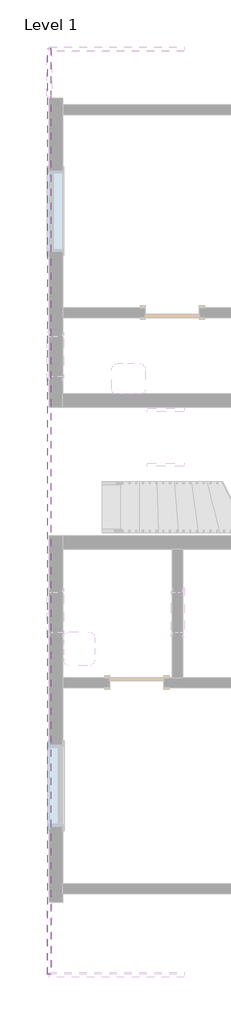
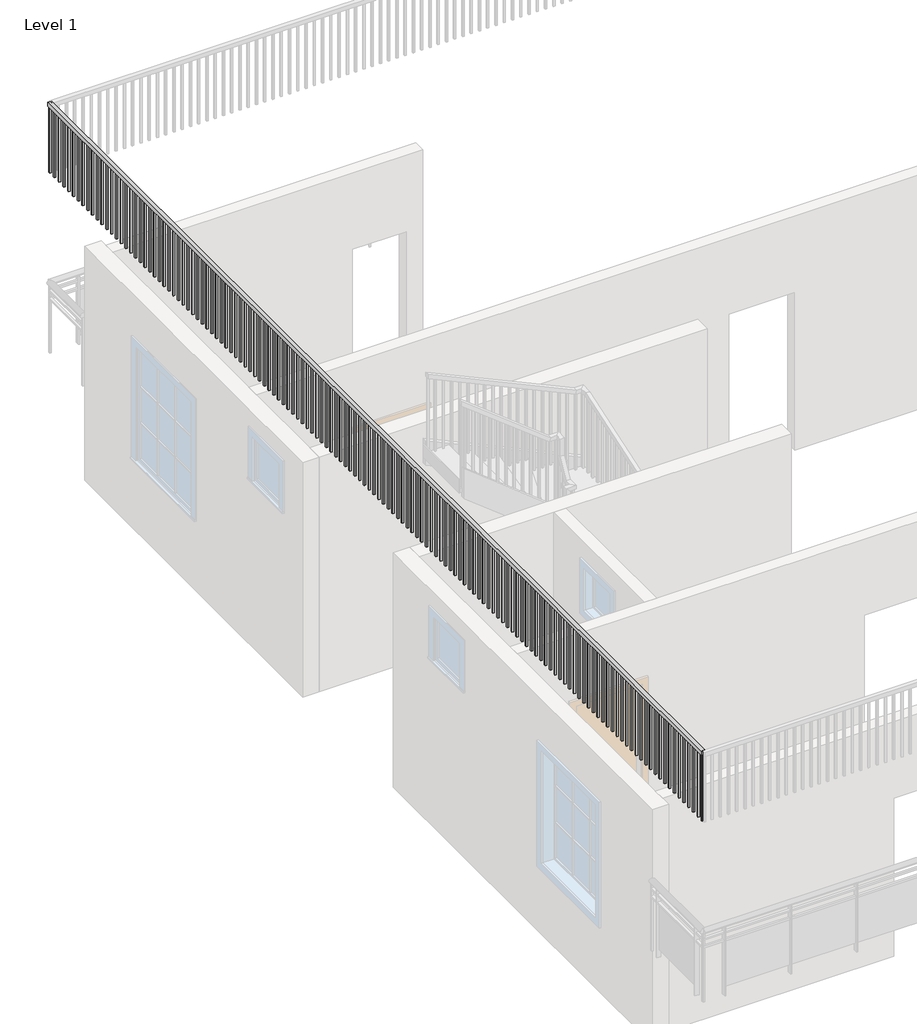
# One storey, part 3 of 7: 1 railing.
"""IFC4 building model written with IfcOpenShell, lengths in millimetres."""

from ifc_helpers import new_model, si_unit, frame, origin, place, context, project, spatial, polyline, outline, extrude, element, save

model = new_model("IFC4")

# Units and contexts
model_context = context("Model", 3, world=origin())
ifc_project = project(units=[si_unit("LENGTHUNIT", "METRE", prefix="MILLI")], contexts=[model_context])

# Site, building, storey
site = spatial("IfcSite", under=ifc_project)
building = spatial("IfcBuilding", under=site)
storey = spatial("IfcBuildingStorey", under=building, Name="Level 1", Elevation=0.0)

# Railing
placement = place(None, origin())
element("IfcRailing", 1, ObjectType="Handrail - Rectangular", at=placement, inside=storey, context=model_context, shape_type="SweptSolid", body=[
    extrude(outline(polyline([(-8502.50975, 12460.2089473), (-8451.70975, 12460.2089473), (-8451.70975, -1458.9910527), (-8502.50975, -1458.9910527), (-8502.50975, 12460.2089473)])), frame((0.0, 0.0, 4419.6), z_axis=(0.0, 0.0, 1.0), x_axis=(1.0, 0.0, 0.0)), (0.0, 0.0, 1.0), 50.8),
    extrude(outline(polyline([(-8486.63475, -1347.8660527), (-8467.58475, -1347.8660527), (-8467.58475, -1366.9160527), (-8486.63475, -1366.9160527), (-8486.63475, -1347.8660527)])), frame((0.0, 0.0, 3556.0), z_axis=(0.0, 0.0, 1.0), x_axis=(1.0, 0.0, 0.0)), (0.0, 0.0, 1.0), 863.6),
    extrude(outline(polyline([(-8486.63475, -1246.2660527), (-8467.58475, -1246.2660527), (-8467.58475, -1265.3160527), (-8486.63475, -1265.3160527), (-8486.63475, -1246.2660527)])), frame((0.0, 0.0, 3556.0), z_axis=(0.0, 0.0, 1.0), x_axis=(1.0, 0.0, 0.0)), (0.0, 0.0, 1.0), 863.6),
    extrude(outline(polyline([(-8486.63475, -1144.6660527), (-8467.58475, -1144.6660527), (-8467.58475, -1163.7160527), (-8486.63475, -1163.7160527), (-8486.63475, -1144.6660527)])), frame((0.0, 0.0, 3556.0), z_axis=(0.0, 0.0, 1.0), x_axis=(1.0, 0.0, 0.0)), (0.0, 0.0, 1.0), 863.6),
    extrude(outline(polyline([(-8486.63475, -1043.0660527), (-8467.58475, -1043.0660527), (-8467.58475, -1062.1160527), (-8486.63475, -1062.1160527), (-8486.63475, -1043.0660527)])), frame((0.0, 0.0, 3556.0), z_axis=(0.0, 0.0, 1.0), x_axis=(1.0, 0.0, 0.0)), (0.0, 0.0, 1.0), 863.6),
    extrude(outline(polyline([(-8486.63475, -941.4660527), (-8467.58475, -941.4660527), (-8467.58475, -960.5160527), (-8486.63475, -960.5160527), (-8486.63475, -941.4660527)])), frame((0.0, 0.0, 3556.0), z_axis=(0.0, 0.0, 1.0), x_axis=(1.0, 0.0, 0.0)), (0.0, 0.0, 1.0), 863.6),
    extrude(outline(polyline([(-8486.63475, -839.8660527), (-8467.58475, -839.8660527), (-8467.58475, -858.9160527), (-8486.63475, -858.9160527), (-8486.63475, -839.8660527)])), frame((0.0, 0.0, 3556.0), z_axis=(0.0, 0.0, 1.0), x_axis=(1.0, 0.0, 0.0)), (0.0, 0.0, 1.0), 863.6),
    extrude(outline(polyline([(-8486.63475, -738.2660527), (-8467.58475, -738.2660527), (-8467.58475, -757.3160527), (-8486.63475, -757.3160527), (-8486.63475, -738.2660527)])), frame((0.0, 0.0, 3556.0), z_axis=(0.0, 0.0, 1.0), x_axis=(1.0, 0.0, 0.0)), (0.0, 0.0, 1.0), 863.6),
    extrude(outline(polyline([(-8486.63475, -636.6660527), (-8467.58475, -636.6660527), (-8467.58475, -655.7160527), (-8486.63475, -655.7160527), (-8486.63475, -636.6660527)])), frame((0.0, 0.0, 3556.0), z_axis=(0.0, 0.0, 1.0), x_axis=(1.0, 0.0, 0.0)), (0.0, 0.0, 1.0), 863.6),
    extrude(outline(polyline([(-8486.63475, -535.0660527), (-8467.58475, -535.0660527), (-8467.58475, -554.1160527), (-8486.63475, -554.1160527), (-8486.63475, -535.0660527)])), frame((0.0, 0.0, 3556.0), z_axis=(0.0, 0.0, 1.0), x_axis=(1.0, 0.0, 0.0)), (0.0, 0.0, 1.0), 863.6),
    extrude(outline(polyline([(-8486.63475, -433.4660527), (-8467.58475, -433.4660527), (-8467.58475, -452.5160527), (-8486.63475, -452.5160527), (-8486.63475, -433.4660527)])), frame((0.0, 0.0, 3556.0), z_axis=(0.0, 0.0, 1.0), x_axis=(1.0, 0.0, 0.0)), (0.0, 0.0, 1.0), 863.6),
    extrude(outline(polyline([(-8486.63475, -331.8660527), (-8467.58475, -331.8660527), (-8467.58475, -350.9160527), (-8486.63475, -350.9160527), (-8486.63475, -331.8660527)])), frame((0.0, 0.0, 3556.0), z_axis=(0.0, 0.0, 1.0), x_axis=(1.0, 0.0, 0.0)), (0.0, 0.0, 1.0), 863.6),
    extrude(outline(polyline([(-8486.63475, -230.2660527), (-8467.58475, -230.2660527), (-8467.58475, -249.3160527), (-8486.63475, -249.3160527), (-8486.63475, -230.2660527)])), frame((0.0, 0.0, 3556.0), z_axis=(0.0, 0.0, 1.0), x_axis=(1.0, 0.0, 0.0)), (0.0, 0.0, 1.0), 863.6),
    extrude(outline(polyline([(-8486.63475, -128.6660527), (-8467.58475, -128.6660527), (-8467.58475, -147.7160527), (-8486.63475, -147.7160527), (-8486.63475, -128.6660527)])), frame((0.0, 0.0, 3556.0), z_axis=(0.0, 0.0, 1.0), x_axis=(1.0, 0.0, 0.0)), (0.0, 0.0, 1.0), 863.6),
    extrude(outline(polyline([(-8486.63475, -27.0660527), (-8467.58475, -27.0660527), (-8467.58475, -46.1160527), (-8486.63475, -46.1160527), (-8486.63475, -27.0660527)])), frame((0.0, 0.0, 3556.0), z_axis=(0.0, 0.0, 1.0), x_axis=(1.0, 0.0, 0.0)), (0.0, 0.0, 1.0), 863.6),
    extrude(outline(polyline([(-8486.63475, 74.5339473), (-8467.58475, 74.5339473), (-8467.58475, 55.4839473), (-8486.63475, 55.4839473), (-8486.63475, 74.5339473)])), frame((0.0, 0.0, 3556.0), z_axis=(0.0, 0.0, 1.0), x_axis=(1.0, 0.0, 0.0)), (0.0, 0.0, 1.0), 863.6),
    extrude(outline(polyline([(-8486.63475, 176.1339473), (-8467.58475, 176.1339473), (-8467.58475, 157.0839473), (-8486.63475, 157.0839473), (-8486.63475, 176.1339473)])), frame((0.0, 0.0, 3556.0), z_axis=(0.0, 0.0, 1.0), x_axis=(1.0, 0.0, 0.0)), (0.0, 0.0, 1.0), 863.6),
    extrude(outline(polyline([(-8486.63475, 277.7339473), (-8467.58475, 277.7339473), (-8467.58475, 258.6839473), (-8486.63475, 258.6839473), (-8486.63475, 277.7339473)])), frame((0.0, 0.0, 3556.0), z_axis=(0.0, 0.0, 1.0), x_axis=(1.0, 0.0, 0.0)), (0.0, 0.0, 1.0), 863.6),
    extrude(outline(polyline([(-8486.63475, 379.3339473), (-8467.58475, 379.3339473), (-8467.58475, 360.2839473), (-8486.63475, 360.2839473), (-8486.63475, 379.3339473)])), frame((0.0, 0.0, 3556.0), z_axis=(0.0, 0.0, 1.0), x_axis=(1.0, 0.0, 0.0)), (0.0, 0.0, 1.0), 863.6),
    extrude(outline(polyline([(-8486.63475, 480.9339473), (-8467.58475, 480.9339473), (-8467.58475, 461.8839473), (-8486.63475, 461.8839473), (-8486.63475, 480.9339473)])), frame((0.0, 0.0, 3556.0), z_axis=(0.0, 0.0, 1.0), x_axis=(1.0, 0.0, 0.0)), (0.0, 0.0, 1.0), 863.6),
    extrude(outline(polyline([(-8486.63475, 582.5339473), (-8467.58475, 582.5339473), (-8467.58475, 563.4839473), (-8486.63475, 563.4839473), (-8486.63475, 582.5339473)])), frame((0.0, 0.0, 3556.0), z_axis=(0.0, 0.0, 1.0), x_axis=(1.0, 0.0, 0.0)), (0.0, 0.0, 1.0), 863.6),
    extrude(outline(polyline([(-8486.63475, 684.1339473), (-8467.58475, 684.1339473), (-8467.58475, 665.0839473), (-8486.63475, 665.0839473), (-8486.63475, 684.1339473)])), frame((0.0, 0.0, 3556.0), z_axis=(0.0, 0.0, 1.0), x_axis=(1.0, 0.0, 0.0)), (0.0, 0.0, 1.0), 863.6),
    extrude(outline(polyline([(-8486.63475, 785.7339473), (-8467.58475, 785.7339473), (-8467.58475, 766.6839473), (-8486.63475, 766.6839473), (-8486.63475, 785.7339473)])), frame((0.0, 0.0, 3556.0), z_axis=(0.0, 0.0, 1.0), x_axis=(1.0, 0.0, 0.0)), (0.0, 0.0, 1.0), 863.6),
    extrude(outline(polyline([(-8486.63475, 887.3339473), (-8467.58475, 887.3339473), (-8467.58475, 868.2839473), (-8486.63475, 868.2839473), (-8486.63475, 887.3339473)])), frame((0.0, 0.0, 3556.0), z_axis=(0.0, 0.0, 1.0), x_axis=(1.0, 0.0, 0.0)), (0.0, 0.0, 1.0), 863.6),
    extrude(outline(polyline([(-8486.63475, 988.9339473), (-8467.58475, 988.9339473), (-8467.58475, 969.8839473), (-8486.63475, 969.8839473), (-8486.63475, 988.9339473)])), frame((0.0, 0.0, 3556.0), z_axis=(0.0, 0.0, 1.0), x_axis=(1.0, 0.0, 0.0)), (0.0, 0.0, 1.0), 863.6),
    extrude(outline(polyline([(-8486.63475, 1090.5339473), (-8467.58475, 1090.5339473), (-8467.58475, 1071.4839473), (-8486.63475, 1071.4839473), (-8486.63475, 1090.5339473)])), frame((0.0, 0.0, 3556.0), z_axis=(0.0, 0.0, 1.0), x_axis=(1.0, 0.0, 0.0)), (0.0, 0.0, 1.0), 863.6),
    extrude(outline(polyline([(-8486.63475, 1192.1339473), (-8467.58475, 1192.1339473), (-8467.58475, 1173.0839473), (-8486.63475, 1173.0839473), (-8486.63475, 1192.1339473)])), frame((0.0, 0.0, 3556.0), z_axis=(0.0, 0.0, 1.0), x_axis=(1.0, 0.0, 0.0)), (0.0, 0.0, 1.0), 863.6),
    extrude(outline(polyline([(-8486.63475, 1293.7339473), (-8467.58475, 1293.7339473), (-8467.58475, 1274.6839473), (-8486.63475, 1274.6839473), (-8486.63475, 1293.7339473)])), frame((0.0, 0.0, 3556.0), z_axis=(0.0, 0.0, 1.0), x_axis=(1.0, 0.0, 0.0)), (0.0, 0.0, 1.0), 863.6),
    extrude(outline(polyline([(-8486.63475, 1395.3339473), (-8467.58475, 1395.3339473), (-8467.58475, 1376.2839473), (-8486.63475, 1376.2839473), (-8486.63475, 1395.3339473)])), frame((0.0, 0.0, 3556.0), z_axis=(0.0, 0.0, 1.0), x_axis=(1.0, 0.0, 0.0)), (0.0, 0.0, 1.0), 863.6),
    extrude(outline(polyline([(-8486.63475, 1496.9339473), (-8467.58475, 1496.9339473), (-8467.58475, 1477.8839473), (-8486.63475, 1477.8839473), (-8486.63475, 1496.9339473)])), frame((0.0, 0.0, 3556.0), z_axis=(0.0, 0.0, 1.0), x_axis=(1.0, 0.0, 0.0)), (0.0, 0.0, 1.0), 863.6),
    extrude(outline(polyline([(-8486.63475, 1598.5339473), (-8467.58475, 1598.5339473), (-8467.58475, 1579.4839473), (-8486.63475, 1579.4839473), (-8486.63475, 1598.5339473)])), frame((0.0, 0.0, 3556.0), z_axis=(0.0, 0.0, 1.0), x_axis=(1.0, 0.0, 0.0)), (0.0, 0.0, 1.0), 863.6),
    extrude(outline(polyline([(-8486.63475, 1700.1339473), (-8467.58475, 1700.1339473), (-8467.58475, 1681.0839473), (-8486.63475, 1681.0839473), (-8486.63475, 1700.1339473)])), frame((0.0, 0.0, 3556.0), z_axis=(0.0, 0.0, 1.0), x_axis=(1.0, 0.0, 0.0)), (0.0, 0.0, 1.0), 863.6),
    extrude(outline(polyline([(-8486.63475, 1801.7339473), (-8467.58475, 1801.7339473), (-8467.58475, 1782.6839473), (-8486.63475, 1782.6839473), (-8486.63475, 1801.7339473)])), frame((0.0, 0.0, 3556.0), z_axis=(0.0, 0.0, 1.0), x_axis=(1.0, 0.0, 0.0)), (0.0, 0.0, 1.0), 863.6),
    extrude(outline(polyline([(-8486.63475, 1903.3339473), (-8467.58475, 1903.3339473), (-8467.58475, 1884.2839473), (-8486.63475, 1884.2839473), (-8486.63475, 1903.3339473)])), frame((0.0, 0.0, 3556.0), z_axis=(0.0, 0.0, 1.0), x_axis=(1.0, 0.0, 0.0)), (0.0, 0.0, 1.0), 863.6),
    extrude(outline(polyline([(-8486.63475, 2004.9339473), (-8467.58475, 2004.9339473), (-8467.58475, 1985.8839473), (-8486.63475, 1985.8839473), (-8486.63475, 2004.9339473)])), frame((0.0, 0.0, 3556.0), z_axis=(0.0, 0.0, 1.0), x_axis=(1.0, 0.0, 0.0)), (0.0, 0.0, 1.0), 863.6),
    extrude(outline(polyline([(-8486.63475, 2106.5339473), (-8467.58475, 2106.5339473), (-8467.58475, 2087.4839473), (-8486.63475, 2087.4839473), (-8486.63475, 2106.5339473)])), frame((0.0, 0.0, 3556.0), z_axis=(0.0, 0.0, 1.0), x_axis=(1.0, 0.0, 0.0)), (0.0, 0.0, 1.0), 863.6),
    extrude(outline(polyline([(-8486.63475, 2208.1339473), (-8467.58475, 2208.1339473), (-8467.58475, 2189.0839473), (-8486.63475, 2189.0839473), (-8486.63475, 2208.1339473)])), frame((0.0, 0.0, 3556.0), z_axis=(0.0, 0.0, 1.0), x_axis=(1.0, 0.0, 0.0)), (0.0, 0.0, 1.0), 863.6),
    extrude(outline(polyline([(-8486.63475, 2309.7339473), (-8467.58475, 2309.7339473), (-8467.58475, 2290.6839473), (-8486.63475, 2290.6839473), (-8486.63475, 2309.7339473)])), frame((0.0, 0.0, 3556.0), z_axis=(0.0, 0.0, 1.0), x_axis=(1.0, 0.0, 0.0)), (0.0, 0.0, 1.0), 863.6),
    extrude(outline(polyline([(-8486.63475, 2411.3339473), (-8467.58475, 2411.3339473), (-8467.58475, 2392.2839473), (-8486.63475, 2392.2839473), (-8486.63475, 2411.3339473)])), frame((0.0, 0.0, 3556.0), z_axis=(0.0, 0.0, 1.0), x_axis=(1.0, 0.0, 0.0)), (0.0, 0.0, 1.0), 863.6),
    extrude(outline(polyline([(-8486.63475, 2512.9339473), (-8467.58475, 2512.9339473), (-8467.58475, 2493.8839473), (-8486.63475, 2493.8839473), (-8486.63475, 2512.9339473)])), frame((0.0, 0.0, 3556.0), z_axis=(0.0, 0.0, 1.0), x_axis=(1.0, 0.0, 0.0)), (0.0, 0.0, 1.0), 863.6),
    extrude(outline(polyline([(-8486.63475, 2614.5339473), (-8467.58475, 2614.5339473), (-8467.58475, 2595.4839473), (-8486.63475, 2595.4839473), (-8486.63475, 2614.5339473)])), frame((0.0, 0.0, 3556.0), z_axis=(0.0, 0.0, 1.0), x_axis=(1.0, 0.0, 0.0)), (0.0, 0.0, 1.0), 863.6),
    extrude(outline(polyline([(-8486.63475, 2716.1339473), (-8467.58475, 2716.1339473), (-8467.58475, 2697.0839473), (-8486.63475, 2697.0839473), (-8486.63475, 2716.1339473)])), frame((0.0, 0.0, 3556.0), z_axis=(0.0, 0.0, 1.0), x_axis=(1.0, 0.0, 0.0)), (0.0, 0.0, 1.0), 863.6),
    extrude(outline(polyline([(-8486.63475, 2817.7339473), (-8467.58475, 2817.7339473), (-8467.58475, 2798.6839473), (-8486.63475, 2798.6839473), (-8486.63475, 2817.7339473)])), frame((0.0, 0.0, 3556.0), z_axis=(0.0, 0.0, 1.0), x_axis=(1.0, 0.0, 0.0)), (0.0, 0.0, 1.0), 863.6),
    extrude(outline(polyline([(-8486.63475, 2919.3339473), (-8467.58475, 2919.3339473), (-8467.58475, 2900.2839473), (-8486.63475, 2900.2839473), (-8486.63475, 2919.3339473)])), frame((0.0, 0.0, 3556.0), z_axis=(0.0, 0.0, 1.0), x_axis=(1.0, 0.0, 0.0)), (0.0, 0.0, 1.0), 863.6),
    extrude(outline(polyline([(-8486.63475, 3020.9339473), (-8467.58475, 3020.9339473), (-8467.58475, 3001.8839473), (-8486.63475, 3001.8839473), (-8486.63475, 3020.9339473)])), frame((0.0, 0.0, 3556.0), z_axis=(0.0, 0.0, 1.0), x_axis=(1.0, 0.0, 0.0)), (0.0, 0.0, 1.0), 863.6),
    extrude(outline(polyline([(-8486.63475, 3122.5339473), (-8467.58475, 3122.5339473), (-8467.58475, 3103.4839473), (-8486.63475, 3103.4839473), (-8486.63475, 3122.5339473)])), frame((0.0, 0.0, 3556.0), z_axis=(0.0, 0.0, 1.0), x_axis=(1.0, 0.0, 0.0)), (0.0, 0.0, 1.0), 863.6),
    extrude(outline(polyline([(-8486.63475, 3224.1339473), (-8467.58475, 3224.1339473), (-8467.58475, 3205.0839473), (-8486.63475, 3205.0839473), (-8486.63475, 3224.1339473)])), frame((0.0, 0.0, 3556.0), z_axis=(0.0, 0.0, 1.0), x_axis=(1.0, 0.0, 0.0)), (0.0, 0.0, 1.0), 863.6),
    extrude(outline(polyline([(-8486.63475, 3325.7339473), (-8467.58475, 3325.7339473), (-8467.58475, 3306.6839473), (-8486.63475, 3306.6839473), (-8486.63475, 3325.7339473)])), frame((0.0, 0.0, 3556.0), z_axis=(0.0, 0.0, 1.0), x_axis=(1.0, 0.0, 0.0)), (0.0, 0.0, 1.0), 863.6),
    extrude(outline(polyline([(-8486.63475, 3427.3339473), (-8467.58475, 3427.3339473), (-8467.58475, 3408.2839473), (-8486.63475, 3408.2839473), (-8486.63475, 3427.3339473)])), frame((0.0, 0.0, 3556.0), z_axis=(0.0, 0.0, 1.0), x_axis=(1.0, 0.0, 0.0)), (0.0, 0.0, 1.0), 863.6),
    extrude(outline(polyline([(-8486.63475, 3528.9339473), (-8467.58475, 3528.9339473), (-8467.58475, 3509.8839473), (-8486.63475, 3509.8839473), (-8486.63475, 3528.9339473)])), frame((0.0, 0.0, 3556.0), z_axis=(0.0, 0.0, 1.0), x_axis=(1.0, 0.0, 0.0)), (0.0, 0.0, 1.0), 863.6),
    extrude(outline(polyline([(-8486.63475, 3630.5339473), (-8467.58475, 3630.5339473), (-8467.58475, 3611.4839473), (-8486.63475, 3611.4839473), (-8486.63475, 3630.5339473)])), frame((0.0, 0.0, 3556.0), z_axis=(0.0, 0.0, 1.0), x_axis=(1.0, 0.0, 0.0)), (0.0, 0.0, 1.0), 863.6),
    extrude(outline(polyline([(-8486.63475, 3732.1339473), (-8467.58475, 3732.1339473), (-8467.58475, 3713.0839473), (-8486.63475, 3713.0839473), (-8486.63475, 3732.1339473)])), frame((0.0, 0.0, 3556.0), z_axis=(0.0, 0.0, 1.0), x_axis=(1.0, 0.0, 0.0)), (0.0, 0.0, 1.0), 863.6),
    extrude(outline(polyline([(-8486.63475, 3833.7339473), (-8467.58475, 3833.7339473), (-8467.58475, 3814.6839473), (-8486.63475, 3814.6839473), (-8486.63475, 3833.7339473)])), frame((0.0, 0.0, 3556.0), z_axis=(0.0, 0.0, 1.0), x_axis=(1.0, 0.0, 0.0)), (0.0, 0.0, 1.0), 863.6),
    extrude(outline(polyline([(-8486.63475, 3935.3339473), (-8467.58475, 3935.3339473), (-8467.58475, 3916.2839473), (-8486.63475, 3916.2839473), (-8486.63475, 3935.3339473)])), frame((0.0, 0.0, 3556.0), z_axis=(0.0, 0.0, 1.0), x_axis=(1.0, 0.0, 0.0)), (0.0, 0.0, 1.0), 863.6),
    extrude(outline(polyline([(-8486.63475, 4036.9339473), (-8467.58475, 4036.9339473), (-8467.58475, 4017.8839473), (-8486.63475, 4017.8839473), (-8486.63475, 4036.9339473)])), frame((0.0, 0.0, 3556.0), z_axis=(0.0, 0.0, 1.0), x_axis=(1.0, 0.0, 0.0)), (0.0, 0.0, 1.0), 863.6),
    extrude(outline(polyline([(-8486.63475, 4138.5339473), (-8467.58475, 4138.5339473), (-8467.58475, 4119.4839473), (-8486.63475, 4119.4839473), (-8486.63475, 4138.5339473)])), frame((0.0, 0.0, 3556.0), z_axis=(0.0, 0.0, 1.0), x_axis=(1.0, 0.0, 0.0)), (0.0, 0.0, 1.0), 863.6),
    extrude(outline(polyline([(-8486.63475, 4240.1339473), (-8467.58475, 4240.1339473), (-8467.58475, 4221.0839473), (-8486.63475, 4221.0839473), (-8486.63475, 4240.1339473)])), frame((0.0, 0.0, 3556.0), z_axis=(0.0, 0.0, 1.0), x_axis=(1.0, 0.0, 0.0)), (0.0, 0.0, 1.0), 863.6),
    extrude(outline(polyline([(-8486.63475, 4341.7339473), (-8467.58475, 4341.7339473), (-8467.58475, 4322.6839473), (-8486.63475, 4322.6839473), (-8486.63475, 4341.7339473)])), frame((0.0, 0.0, 3556.0), z_axis=(0.0, 0.0, 1.0), x_axis=(1.0, 0.0, 0.0)), (0.0, 0.0, 1.0), 863.6),
    extrude(outline(polyline([(-8486.63475, 4443.3339473), (-8467.58475, 4443.3339473), (-8467.58475, 4424.2839473), (-8486.63475, 4424.2839473), (-8486.63475, 4443.3339473)])), frame((0.0, 0.0, 3556.0), z_axis=(0.0, 0.0, 1.0), x_axis=(1.0, 0.0, 0.0)), (0.0, 0.0, 1.0), 863.6),
    extrude(outline(polyline([(-8486.63475, 4544.9339473), (-8467.58475, 4544.9339473), (-8467.58475, 4525.8839473), (-8486.63475, 4525.8839473), (-8486.63475, 4544.9339473)])), frame((0.0, 0.0, 3556.0), z_axis=(0.0, 0.0, 1.0), x_axis=(1.0, 0.0, 0.0)), (0.0, 0.0, 1.0), 863.6),
    extrude(outline(polyline([(-8486.63475, 4646.5339473), (-8467.58475, 4646.5339473), (-8467.58475, 4627.4839473), (-8486.63475, 4627.4839473), (-8486.63475, 4646.5339473)])), frame((0.0, 0.0, 3556.0), z_axis=(0.0, 0.0, 1.0), x_axis=(1.0, 0.0, 0.0)), (0.0, 0.0, 1.0), 863.6),
    extrude(outline(polyline([(-8486.63475, 4748.1339473), (-8467.58475, 4748.1339473), (-8467.58475, 4729.0839473), (-8486.63475, 4729.0839473), (-8486.63475, 4748.1339473)])), frame((0.0, 0.0, 3556.0), z_axis=(0.0, 0.0, 1.0), x_axis=(1.0, 0.0, 0.0)), (0.0, 0.0, 1.0), 863.6),
    extrude(outline(polyline([(-8486.63475, 4849.7339473), (-8467.58475, 4849.7339473), (-8467.58475, 4830.6839473), (-8486.63475, 4830.6839473), (-8486.63475, 4849.7339473)])), frame((0.0, 0.0, 3556.0), z_axis=(0.0, 0.0, 1.0), x_axis=(1.0, 0.0, 0.0)), (0.0, 0.0, 1.0), 863.6),
    extrude(outline(polyline([(-8486.63475, 4951.3339473), (-8467.58475, 4951.3339473), (-8467.58475, 4932.2839473), (-8486.63475, 4932.2839473), (-8486.63475, 4951.3339473)])), frame((0.0, 0.0, 3556.0), z_axis=(0.0, 0.0, 1.0), x_axis=(1.0, 0.0, 0.0)), (0.0, 0.0, 1.0), 863.6),
    extrude(outline(polyline([(-8486.63475, 5052.9339473), (-8467.58475, 5052.9339473), (-8467.58475, 5033.8839473), (-8486.63475, 5033.8839473), (-8486.63475, 5052.9339473)])), frame((0.0, 0.0, 3556.0), z_axis=(0.0, 0.0, 1.0), x_axis=(1.0, 0.0, 0.0)), (0.0, 0.0, 1.0), 863.6),
    extrude(outline(polyline([(-8486.63475, 5154.5339473), (-8467.58475, 5154.5339473), (-8467.58475, 5135.4839473), (-8486.63475, 5135.4839473), (-8486.63475, 5154.5339473)])), frame((0.0, 0.0, 3556.0), z_axis=(0.0, 0.0, 1.0), x_axis=(1.0, 0.0, 0.0)), (0.0, 0.0, 1.0), 863.6),
    extrude(outline(polyline([(-8486.63475, 5256.1339473), (-8467.58475, 5256.1339473), (-8467.58475, 5237.0839473), (-8486.63475, 5237.0839473), (-8486.63475, 5256.1339473)])), frame((0.0, 0.0, 3556.0), z_axis=(0.0, 0.0, 1.0), x_axis=(1.0, 0.0, 0.0)), (0.0, 0.0, 1.0), 863.6),
    extrude(outline(polyline([(-8486.63475, 5357.7339473), (-8467.58475, 5357.7339473), (-8467.58475, 5338.6839473), (-8486.63475, 5338.6839473), (-8486.63475, 5357.7339473)])), frame((0.0, 0.0, 3556.0), z_axis=(0.0, 0.0, 1.0), x_axis=(1.0, 0.0, 0.0)), (0.0, 0.0, 1.0), 863.6),
    extrude(outline(polyline([(-8486.63475, 5459.3339473), (-8467.58475, 5459.3339473), (-8467.58475, 5440.2839473), (-8486.63475, 5440.2839473), (-8486.63475, 5459.3339473)])), frame((0.0, 0.0, 3556.0), z_axis=(0.0, 0.0, 1.0), x_axis=(1.0, 0.0, 0.0)), (0.0, 0.0, 1.0), 863.6),
    extrude(outline(polyline([(-8486.63475, 5560.9339473), (-8467.58475, 5560.9339473), (-8467.58475, 5541.8839473), (-8486.63475, 5541.8839473), (-8486.63475, 5560.9339473)])), frame((0.0, 0.0, 3556.0), z_axis=(0.0, 0.0, 1.0), x_axis=(1.0, 0.0, 0.0)), (0.0, 0.0, 1.0), 863.6),
    extrude(outline(polyline([(-8486.63475, 5662.5339473), (-8467.58475, 5662.5339473), (-8467.58475, 5643.4839473), (-8486.63475, 5643.4839473), (-8486.63475, 5662.5339473)])), frame((0.0, 0.0, 3556.0), z_axis=(0.0, 0.0, 1.0), x_axis=(1.0, 0.0, 0.0)), (0.0, 0.0, 1.0), 863.6),
    extrude(outline(polyline([(-8486.63475, 5764.1339473), (-8467.58475, 5764.1339473), (-8467.58475, 5745.0839473), (-8486.63475, 5745.0839473), (-8486.63475, 5764.1339473)])), frame((0.0, 0.0, 3556.0), z_axis=(0.0, 0.0, 1.0), x_axis=(1.0, 0.0, 0.0)), (0.0, 0.0, 1.0), 863.6),
    extrude(outline(polyline([(-8486.63475, 5865.7339473), (-8467.58475, 5865.7339473), (-8467.58475, 5846.6839473), (-8486.63475, 5846.6839473), (-8486.63475, 5865.7339473)])), frame((0.0, 0.0, 3556.0), z_axis=(0.0, 0.0, 1.0), x_axis=(1.0, 0.0, 0.0)), (0.0, 0.0, 1.0), 863.6),
    extrude(outline(polyline([(-8486.63475, 5967.3339473), (-8467.58475, 5967.3339473), (-8467.58475, 5948.2839473), (-8486.63475, 5948.2839473), (-8486.63475, 5967.3339473)])), frame((0.0, 0.0, 3556.0), z_axis=(0.0, 0.0, 1.0), x_axis=(1.0, 0.0, 0.0)), (0.0, 0.0, 1.0), 863.6),
    extrude(outline(polyline([(-8486.63475, 6068.9339473), (-8467.58475, 6068.9339473), (-8467.58475, 6049.8839473), (-8486.63475, 6049.8839473), (-8486.63475, 6068.9339473)])), frame((0.0, 0.0, 3556.0), z_axis=(0.0, 0.0, 1.0), x_axis=(1.0, 0.0, 0.0)), (0.0, 0.0, 1.0), 863.6),
    extrude(outline(polyline([(-8486.63475, 6170.5339473), (-8467.58475, 6170.5339473), (-8467.58475, 6151.4839473), (-8486.63475, 6151.4839473), (-8486.63475, 6170.5339473)])), frame((0.0, 0.0, 3556.0), z_axis=(0.0, 0.0, 1.0), x_axis=(1.0, 0.0, 0.0)), (0.0, 0.0, 1.0), 863.6),
    extrude(outline(polyline([(-8486.63475, 6272.1339473), (-8467.58475, 6272.1339473), (-8467.58475, 6253.0839473), (-8486.63475, 6253.0839473), (-8486.63475, 6272.1339473)])), frame((0.0, 0.0, 3556.0), z_axis=(0.0, 0.0, 1.0), x_axis=(1.0, 0.0, 0.0)), (0.0, 0.0, 1.0), 863.6),
    extrude(outline(polyline([(-8486.63475, 6373.7339473), (-8467.58475, 6373.7339473), (-8467.58475, 6354.6839473), (-8486.63475, 6354.6839473), (-8486.63475, 6373.7339473)])), frame((0.0, 0.0, 3556.0), z_axis=(0.0, 0.0, 1.0), x_axis=(1.0, 0.0, 0.0)), (0.0, 0.0, 1.0), 863.6),
    extrude(outline(polyline([(-8486.63475, 6475.3339473), (-8467.58475, 6475.3339473), (-8467.58475, 6456.2839473), (-8486.63475, 6456.2839473), (-8486.63475, 6475.3339473)])), frame((0.0, 0.0, 3556.0), z_axis=(0.0, 0.0, 1.0), x_axis=(1.0, 0.0, 0.0)), (0.0, 0.0, 1.0), 863.6),
    extrude(outline(polyline([(-8486.63475, 6576.9339473), (-8467.58475, 6576.9339473), (-8467.58475, 6557.8839473), (-8486.63475, 6557.8839473), (-8486.63475, 6576.9339473)])), frame((0.0, 0.0, 3556.0), z_axis=(0.0, 0.0, 1.0), x_axis=(1.0, 0.0, 0.0)), (0.0, 0.0, 1.0), 863.6),
    extrude(outline(polyline([(-8486.63475, 6678.5339473), (-8467.58475, 6678.5339473), (-8467.58475, 6659.4839473), (-8486.63475, 6659.4839473), (-8486.63475, 6678.5339473)])), frame((0.0, 0.0, 3556.0), z_axis=(0.0, 0.0, 1.0), x_axis=(1.0, 0.0, 0.0)), (0.0, 0.0, 1.0), 863.6),
    extrude(outline(polyline([(-8486.63475, 6780.1339473), (-8467.58475, 6780.1339473), (-8467.58475, 6761.0839473), (-8486.63475, 6761.0839473), (-8486.63475, 6780.1339473)])), frame((0.0, 0.0, 3556.0), z_axis=(0.0, 0.0, 1.0), x_axis=(1.0, 0.0, 0.0)), (0.0, 0.0, 1.0), 863.6),
    extrude(outline(polyline([(-8486.63475, 6881.7339473), (-8467.58475, 6881.7339473), (-8467.58475, 6862.6839473), (-8486.63475, 6862.6839473), (-8486.63475, 6881.7339473)])), frame((0.0, 0.0, 3556.0), z_axis=(0.0, 0.0, 1.0), x_axis=(1.0, 0.0, 0.0)), (0.0, 0.0, 1.0), 863.6),
    extrude(outline(polyline([(-8486.63475, 6983.3339473), (-8467.58475, 6983.3339473), (-8467.58475, 6964.2839473), (-8486.63475, 6964.2839473), (-8486.63475, 6983.3339473)])), frame((0.0, 0.0, 3556.0), z_axis=(0.0, 0.0, 1.0), x_axis=(1.0, 0.0, 0.0)), (0.0, 0.0, 1.0), 863.6),
    extrude(outline(polyline([(-8486.63475, 7084.9339473), (-8467.58475, 7084.9339473), (-8467.58475, 7065.8839473), (-8486.63475, 7065.8839473), (-8486.63475, 7084.9339473)])), frame((0.0, 0.0, 3556.0), z_axis=(0.0, 0.0, 1.0), x_axis=(1.0, 0.0, 0.0)), (0.0, 0.0, 1.0), 863.6),
    extrude(outline(polyline([(-8486.63475, 7186.5339473), (-8467.58475, 7186.5339473), (-8467.58475, 7167.4839473), (-8486.63475, 7167.4839473), (-8486.63475, 7186.5339473)])), frame((0.0, 0.0, 3556.0), z_axis=(0.0, 0.0, 1.0), x_axis=(1.0, 0.0, 0.0)), (0.0, 0.0, 1.0), 863.6),
    extrude(outline(polyline([(-8486.63475, 7288.1339473), (-8467.58475, 7288.1339473), (-8467.58475, 7269.0839473), (-8486.63475, 7269.0839473), (-8486.63475, 7288.1339473)])), frame((0.0, 0.0, 3556.0), z_axis=(0.0, 0.0, 1.0), x_axis=(1.0, 0.0, 0.0)), (0.0, 0.0, 1.0), 863.6),
    extrude(outline(polyline([(-8486.63475, 7389.7339473), (-8467.58475, 7389.7339473), (-8467.58475, 7370.6839473), (-8486.63475, 7370.6839473), (-8486.63475, 7389.7339473)])), frame((0.0, 0.0, 3556.0), z_axis=(0.0, 0.0, 1.0), x_axis=(1.0, 0.0, 0.0)), (0.0, 0.0, 1.0), 863.6),
    extrude(outline(polyline([(-8486.63475, 7491.3339473), (-8467.58475, 7491.3339473), (-8467.58475, 7472.2839473), (-8486.63475, 7472.2839473), (-8486.63475, 7491.3339473)])), frame((0.0, 0.0, 3556.0), z_axis=(0.0, 0.0, 1.0), x_axis=(1.0, 0.0, 0.0)), (0.0, 0.0, 1.0), 863.6),
    extrude(outline(polyline([(-8486.63475, 7592.9339473), (-8467.58475, 7592.9339473), (-8467.58475, 7573.8839473), (-8486.63475, 7573.8839473), (-8486.63475, 7592.9339473)])), frame((0.0, 0.0, 3556.0), z_axis=(0.0, 0.0, 1.0), x_axis=(1.0, 0.0, 0.0)), (0.0, 0.0, 1.0), 863.6),
    extrude(outline(polyline([(-8486.63475, 7694.5339473), (-8467.58475, 7694.5339473), (-8467.58475, 7675.4839473), (-8486.63475, 7675.4839473), (-8486.63475, 7694.5339473)])), frame((0.0, 0.0, 3556.0), z_axis=(0.0, 0.0, 1.0), x_axis=(1.0, 0.0, 0.0)), (0.0, 0.0, 1.0), 863.6),
    extrude(outline(polyline([(-8486.63475, 7796.1339473), (-8467.58475, 7796.1339473), (-8467.58475, 7777.0839473), (-8486.63475, 7777.0839473), (-8486.63475, 7796.1339473)])), frame((0.0, 0.0, 3556.0), z_axis=(0.0, 0.0, 1.0), x_axis=(1.0, 0.0, 0.0)), (0.0, 0.0, 1.0), 863.6),
    extrude(outline(polyline([(-8486.63475, 7897.7339473), (-8467.58475, 7897.7339473), (-8467.58475, 7878.6839473), (-8486.63475, 7878.6839473), (-8486.63475, 7897.7339473)])), frame((0.0, 0.0, 3556.0), z_axis=(0.0, 0.0, 1.0), x_axis=(1.0, 0.0, 0.0)), (0.0, 0.0, 1.0), 863.6),
    extrude(outline(polyline([(-8486.63475, 7999.3339473), (-8467.58475, 7999.3339473), (-8467.58475, 7980.2839473), (-8486.63475, 7980.2839473), (-8486.63475, 7999.3339473)])), frame((0.0, 0.0, 3556.0), z_axis=(0.0, 0.0, 1.0), x_axis=(1.0, 0.0, 0.0)), (0.0, 0.0, 1.0), 863.6),
    extrude(outline(polyline([(-8486.63475, 8100.9339473), (-8467.58475, 8100.9339473), (-8467.58475, 8081.8839473), (-8486.63475, 8081.8839473), (-8486.63475, 8100.9339473)])), frame((0.0, 0.0, 3556.0), z_axis=(0.0, 0.0, 1.0), x_axis=(1.0, 0.0, 0.0)), (0.0, 0.0, 1.0), 863.6),
    extrude(outline(polyline([(-8486.63475, 8202.5339473), (-8467.58475, 8202.5339473), (-8467.58475, 8183.4839473), (-8486.63475, 8183.4839473), (-8486.63475, 8202.5339473)])), frame((0.0, 0.0, 3556.0), z_axis=(0.0, 0.0, 1.0), x_axis=(1.0, 0.0, 0.0)), (0.0, 0.0, 1.0), 863.6),
    extrude(outline(polyline([(-8486.63475, 8304.1339473), (-8467.58475, 8304.1339473), (-8467.58475, 8285.0839473), (-8486.63475, 8285.0839473), (-8486.63475, 8304.1339473)])), frame((0.0, 0.0, 3556.0), z_axis=(0.0, 0.0, 1.0), x_axis=(1.0, 0.0, 0.0)), (0.0, 0.0, 1.0), 863.6),
    extrude(outline(polyline([(-8486.63475, 8405.7339473), (-8467.58475, 8405.7339473), (-8467.58475, 8386.6839473), (-8486.63475, 8386.6839473), (-8486.63475, 8405.7339473)])), frame((0.0, 0.0, 3556.0), z_axis=(0.0, 0.0, 1.0), x_axis=(1.0, 0.0, 0.0)), (0.0, 0.0, 1.0), 863.6),
    extrude(outline(polyline([(-8486.63475, 8507.3339473), (-8467.58475, 8507.3339473), (-8467.58475, 8488.2839473), (-8486.63475, 8488.2839473), (-8486.63475, 8507.3339473)])), frame((0.0, 0.0, 3556.0), z_axis=(0.0, 0.0, 1.0), x_axis=(1.0, 0.0, 0.0)), (0.0, 0.0, 1.0), 863.6),
    extrude(outline(polyline([(-8486.63475, 8608.9339473), (-8467.58475, 8608.9339473), (-8467.58475, 8589.8839473), (-8486.63475, 8589.8839473), (-8486.63475, 8608.9339473)])), frame((0.0, 0.0, 3556.0), z_axis=(0.0, 0.0, 1.0), x_axis=(1.0, 0.0, 0.0)), (0.0, 0.0, 1.0), 863.6),
    extrude(outline(polyline([(-8486.63475, 8710.5339473), (-8467.58475, 8710.5339473), (-8467.58475, 8691.4839473), (-8486.63475, 8691.4839473), (-8486.63475, 8710.5339473)])), frame((0.0, 0.0, 3556.0), z_axis=(0.0, 0.0, 1.0), x_axis=(1.0, 0.0, 0.0)), (0.0, 0.0, 1.0), 863.6),
    extrude(outline(polyline([(-8486.63475, 8812.1339473), (-8467.58475, 8812.1339473), (-8467.58475, 8793.0839473), (-8486.63475, 8793.0839473), (-8486.63475, 8812.1339473)])), frame((0.0, 0.0, 3556.0), z_axis=(0.0, 0.0, 1.0), x_axis=(1.0, 0.0, 0.0)), (0.0, 0.0, 1.0), 863.6),
    extrude(outline(polyline([(-8486.63475, 8913.7339473), (-8467.58475, 8913.7339473), (-8467.58475, 8894.6839473), (-8486.63475, 8894.6839473), (-8486.63475, 8913.7339473)])), frame((0.0, 0.0, 3556.0), z_axis=(0.0, 0.0, 1.0), x_axis=(1.0, 0.0, 0.0)), (0.0, 0.0, 1.0), 863.6),
    extrude(outline(polyline([(-8486.63475, 9015.3339473), (-8467.58475, 9015.3339473), (-8467.58475, 8996.2839473), (-8486.63475, 8996.2839473), (-8486.63475, 9015.3339473)])), frame((0.0, 0.0, 3556.0), z_axis=(0.0, 0.0, 1.0), x_axis=(1.0, 0.0, 0.0)), (0.0, 0.0, 1.0), 863.6),
    extrude(outline(polyline([(-8486.63475, 9116.9339473), (-8467.58475, 9116.9339473), (-8467.58475, 9097.8839473), (-8486.63475, 9097.8839473), (-8486.63475, 9116.9339473)])), frame((0.0, 0.0, 3556.0), z_axis=(0.0, 0.0, 1.0), x_axis=(1.0, 0.0, 0.0)), (0.0, 0.0, 1.0), 863.6),
    extrude(outline(polyline([(-8486.63475, 9218.5339473), (-8467.58475, 9218.5339473), (-8467.58475, 9199.4839473), (-8486.63475, 9199.4839473), (-8486.63475, 9218.5339473)])), frame((0.0, 0.0, 3556.0), z_axis=(0.0, 0.0, 1.0), x_axis=(1.0, 0.0, 0.0)), (0.0, 0.0, 1.0), 863.6),
    extrude(outline(polyline([(-8486.63475, 9320.1339473), (-8467.58475, 9320.1339473), (-8467.58475, 9301.0839473), (-8486.63475, 9301.0839473), (-8486.63475, 9320.1339473)])), frame((0.0, 0.0, 3556.0), z_axis=(0.0, 0.0, 1.0), x_axis=(1.0, 0.0, 0.0)), (0.0, 0.0, 1.0), 863.6),
    extrude(outline(polyline([(-8486.63475, 9421.7339473), (-8467.58475, 9421.7339473), (-8467.58475, 9402.6839473), (-8486.63475, 9402.6839473), (-8486.63475, 9421.7339473)])), frame((0.0, 0.0, 3556.0), z_axis=(0.0, 0.0, 1.0), x_axis=(1.0, 0.0, 0.0)), (0.0, 0.0, 1.0), 863.6),
    extrude(outline(polyline([(-8486.63475, 9523.3339473), (-8467.58475, 9523.3339473), (-8467.58475, 9504.2839473), (-8486.63475, 9504.2839473), (-8486.63475, 9523.3339473)])), frame((0.0, 0.0, 3556.0), z_axis=(0.0, 0.0, 1.0), x_axis=(1.0, 0.0, 0.0)), (0.0, 0.0, 1.0), 863.6),
    extrude(outline(polyline([(-8486.63475, 9624.9339473), (-8467.58475, 9624.9339473), (-8467.58475, 9605.8839473), (-8486.63475, 9605.8839473), (-8486.63475, 9624.9339473)])), frame((0.0, 0.0, 3556.0), z_axis=(0.0, 0.0, 1.0), x_axis=(1.0, 0.0, 0.0)), (0.0, 0.0, 1.0), 863.6),
    extrude(outline(polyline([(-8486.63475, 9726.5339473), (-8467.58475, 9726.5339473), (-8467.58475, 9707.4839473), (-8486.63475, 9707.4839473), (-8486.63475, 9726.5339473)])), frame((0.0, 0.0, 3556.0), z_axis=(0.0, 0.0, 1.0), x_axis=(1.0, 0.0, 0.0)), (0.0, 0.0, 1.0), 863.6),
    extrude(outline(polyline([(-8486.63475, 9828.1339473), (-8467.58475, 9828.1339473), (-8467.58475, 9809.0839473), (-8486.63475, 9809.0839473), (-8486.63475, 9828.1339473)])), frame((0.0, 0.0, 3556.0), z_axis=(0.0, 0.0, 1.0), x_axis=(1.0, 0.0, 0.0)), (0.0, 0.0, 1.0), 863.6),
    extrude(outline(polyline([(-8486.63475, 9929.7339473), (-8467.58475, 9929.7339473), (-8467.58475, 9910.6839473), (-8486.63475, 9910.6839473), (-8486.63475, 9929.7339473)])), frame((0.0, 0.0, 3556.0), z_axis=(0.0, 0.0, 1.0), x_axis=(1.0, 0.0, 0.0)), (0.0, 0.0, 1.0), 863.6),
    extrude(outline(polyline([(-8486.63475, 10031.3339473), (-8467.58475, 10031.3339473), (-8467.58475, 10012.2839473), (-8486.63475, 10012.2839473), (-8486.63475, 10031.3339473)])), frame((0.0, 0.0, 3556.0), z_axis=(0.0, 0.0, 1.0), x_axis=(1.0, 0.0, 0.0)), (0.0, 0.0, 1.0), 863.6),
    extrude(outline(polyline([(-8486.63475, 10132.9339473), (-8467.58475, 10132.9339473), (-8467.58475, 10113.8839473), (-8486.63475, 10113.8839473), (-8486.63475, 10132.9339473)])), frame((0.0, 0.0, 3556.0), z_axis=(0.0, 0.0, 1.0), x_axis=(1.0, 0.0, 0.0)), (0.0, 0.0, 1.0), 863.6),
    extrude(outline(polyline([(-8486.63475, 10234.5339473), (-8467.58475, 10234.5339473), (-8467.58475, 10215.4839473), (-8486.63475, 10215.4839473), (-8486.63475, 10234.5339473)])), frame((0.0, 0.0, 3556.0), z_axis=(0.0, 0.0, 1.0), x_axis=(1.0, 0.0, 0.0)), (0.0, 0.0, 1.0), 863.6),
    extrude(outline(polyline([(-8486.63475, 10336.1339473), (-8467.58475, 10336.1339473), (-8467.58475, 10317.0839473), (-8486.63475, 10317.0839473), (-8486.63475, 10336.1339473)])), frame((0.0, 0.0, 3556.0), z_axis=(0.0, 0.0, 1.0), x_axis=(1.0, 0.0, 0.0)), (0.0, 0.0, 1.0), 863.6),
    extrude(outline(polyline([(-8486.63475, 10437.7339473), (-8467.58475, 10437.7339473), (-8467.58475, 10418.6839473), (-8486.63475, 10418.6839473), (-8486.63475, 10437.7339473)])), frame((0.0, 0.0, 3556.0), z_axis=(0.0, 0.0, 1.0), x_axis=(1.0, 0.0, 0.0)), (0.0, 0.0, 1.0), 863.6),
    extrude(outline(polyline([(-8486.63475, 10539.3339473), (-8467.58475, 10539.3339473), (-8467.58475, 10520.2839473), (-8486.63475, 10520.2839473), (-8486.63475, 10539.3339473)])), frame((0.0, 0.0, 3556.0), z_axis=(0.0, 0.0, 1.0), x_axis=(1.0, 0.0, 0.0)), (0.0, 0.0, 1.0), 863.6),
    extrude(outline(polyline([(-8486.63475, 10640.9339473), (-8467.58475, 10640.9339473), (-8467.58475, 10621.8839473), (-8486.63475, 10621.8839473), (-8486.63475, 10640.9339473)])), frame((0.0, 0.0, 3556.0), z_axis=(0.0, 0.0, 1.0), x_axis=(1.0, 0.0, 0.0)), (0.0, 0.0, 1.0), 863.6),
    extrude(outline(polyline([(-8486.63475, 10742.5339473), (-8467.58475, 10742.5339473), (-8467.58475, 10723.4839473), (-8486.63475, 10723.4839473), (-8486.63475, 10742.5339473)])), frame((0.0, 0.0, 3556.0), z_axis=(0.0, 0.0, 1.0), x_axis=(1.0, 0.0, 0.0)), (0.0, 0.0, 1.0), 863.6),
    extrude(outline(polyline([(-8486.63475, 10844.1339473), (-8467.58475, 10844.1339473), (-8467.58475, 10825.0839473), (-8486.63475, 10825.0839473), (-8486.63475, 10844.1339473)])), frame((0.0, 0.0, 3556.0), z_axis=(0.0, 0.0, 1.0), x_axis=(1.0, 0.0, 0.0)), (0.0, 0.0, 1.0), 863.6),
    extrude(outline(polyline([(-8486.63475, 10945.7339473), (-8467.58475, 10945.7339473), (-8467.58475, 10926.6839473), (-8486.63475, 10926.6839473), (-8486.63475, 10945.7339473)])), frame((0.0, 0.0, 3556.0), z_axis=(0.0, 0.0, 1.0), x_axis=(1.0, 0.0, 0.0)), (0.0, 0.0, 1.0), 863.6),
    extrude(outline(polyline([(-8486.63475, 11047.3339473), (-8467.58475, 11047.3339473), (-8467.58475, 11028.2839473), (-8486.63475, 11028.2839473), (-8486.63475, 11047.3339473)])), frame((0.0, 0.0, 3556.0), z_axis=(0.0, 0.0, 1.0), x_axis=(1.0, 0.0, 0.0)), (0.0, 0.0, 1.0), 863.6),
    extrude(outline(polyline([(-8486.63475, 11148.9339473), (-8467.58475, 11148.9339473), (-8467.58475, 11129.8839473), (-8486.63475, 11129.8839473), (-8486.63475, 11148.9339473)])), frame((0.0, 0.0, 3556.0), z_axis=(0.0, 0.0, 1.0), x_axis=(1.0, 0.0, 0.0)), (0.0, 0.0, 1.0), 863.6),
    extrude(outline(polyline([(-8486.63475, 11250.5339473), (-8467.58475, 11250.5339473), (-8467.58475, 11231.4839473), (-8486.63475, 11231.4839473), (-8486.63475, 11250.5339473)])), frame((0.0, 0.0, 3556.0), z_axis=(0.0, 0.0, 1.0), x_axis=(1.0, 0.0, 0.0)), (0.0, 0.0, 1.0), 863.6),
    extrude(outline(polyline([(-8486.63475, 11352.1339473), (-8467.58475, 11352.1339473), (-8467.58475, 11333.0839473), (-8486.63475, 11333.0839473), (-8486.63475, 11352.1339473)])), frame((0.0, 0.0, 3556.0), z_axis=(0.0, 0.0, 1.0), x_axis=(1.0, 0.0, 0.0)), (0.0, 0.0, 1.0), 863.6),
    extrude(outline(polyline([(-8486.63475, 11453.7339473), (-8467.58475, 11453.7339473), (-8467.58475, 11434.6839473), (-8486.63475, 11434.6839473), (-8486.63475, 11453.7339473)])), frame((0.0, 0.0, 3556.0), z_axis=(0.0, 0.0, 1.0), x_axis=(1.0, 0.0, 0.0)), (0.0, 0.0, 1.0), 863.6),
    extrude(outline(polyline([(-8486.63475, 11555.3339473), (-8467.58475, 11555.3339473), (-8467.58475, 11536.2839473), (-8486.63475, 11536.2839473), (-8486.63475, 11555.3339473)])), frame((0.0, 0.0, 3556.0), z_axis=(0.0, 0.0, 1.0), x_axis=(1.0, 0.0, 0.0)), (0.0, 0.0, 1.0), 863.6),
    extrude(outline(polyline([(-8486.63475, 11656.9339473), (-8467.58475, 11656.9339473), (-8467.58475, 11637.8839473), (-8486.63475, 11637.8839473), (-8486.63475, 11656.9339473)])), frame((0.0, 0.0, 3556.0), z_axis=(0.0, 0.0, 1.0), x_axis=(1.0, 0.0, 0.0)), (0.0, 0.0, 1.0), 863.6),
    extrude(outline(polyline([(-8486.63475, 11758.5339473), (-8467.58475, 11758.5339473), (-8467.58475, 11739.4839473), (-8486.63475, 11739.4839473), (-8486.63475, 11758.5339473)])), frame((0.0, 0.0, 3556.0), z_axis=(0.0, 0.0, 1.0), x_axis=(1.0, 0.0, 0.0)), (0.0, 0.0, 1.0), 863.6),
    extrude(outline(polyline([(-8486.63475, 11860.1339473), (-8467.58475, 11860.1339473), (-8467.58475, 11841.0839473), (-8486.63475, 11841.0839473), (-8486.63475, 11860.1339473)])), frame((0.0, 0.0, 3556.0), z_axis=(0.0, 0.0, 1.0), x_axis=(1.0, 0.0, 0.0)), (0.0, 0.0, 1.0), 863.6),
    extrude(outline(polyline([(-8486.63475, 11961.7339473), (-8467.58475, 11961.7339473), (-8467.58475, 11942.6839473), (-8486.63475, 11942.6839473), (-8486.63475, 11961.7339473)])), frame((0.0, 0.0, 3556.0), z_axis=(0.0, 0.0, 1.0), x_axis=(1.0, 0.0, 0.0)), (0.0, 0.0, 1.0), 863.6),
    extrude(outline(polyline([(-8486.63475, 12063.3339473), (-8467.58475, 12063.3339473), (-8467.58475, 12044.2839473), (-8486.63475, 12044.2839473), (-8486.63475, 12063.3339473)])), frame((0.0, 0.0, 3556.0), z_axis=(0.0, 0.0, 1.0), x_axis=(1.0, 0.0, 0.0)), (0.0, 0.0, 1.0), 863.6),
    extrude(outline(polyline([(-8486.63475, 12164.9339473), (-8467.58475, 12164.9339473), (-8467.58475, 12145.8839473), (-8486.63475, 12145.8839473), (-8486.63475, 12164.9339473)])), frame((0.0, 0.0, 3556.0), z_axis=(0.0, 0.0, 1.0), x_axis=(1.0, 0.0, 0.0)), (0.0, 0.0, 1.0), 863.6),
    extrude(outline(polyline([(-8486.63475, 12266.5339473), (-8467.58475, 12266.5339473), (-8467.58475, 12247.4839473), (-8486.63475, 12247.4839473), (-8486.63475, 12266.5339473)])), frame((0.0, 0.0, 3556.0), z_axis=(0.0, 0.0, 1.0), x_axis=(1.0, 0.0, 0.0)), (0.0, 0.0, 1.0), 863.6),
    extrude(outline(polyline([(-8486.63475, 12368.1339473), (-8467.58475, 12368.1339473), (-8467.58475, 12349.0839473), (-8486.63475, 12349.0839473), (-8486.63475, 12368.1339473)])), frame((0.0, 0.0, 3556.0), z_axis=(0.0, 0.0, 1.0), x_axis=(1.0, 0.0, 0.0)), (0.0, 0.0, 1.0), 863.6),
    extrude(outline(polyline([(-8486.63475, -1439.9410527), (-8467.58475, -1439.9410527), (-8467.58475, -1458.9910527), (-8486.63475, -1458.9910527), (-8486.63475, -1439.9410527)])), frame((0.0, 0.0, 3556.0), z_axis=(0.0, 0.0, 1.0), x_axis=(1.0, 0.0, 0.0)), (0.0, 0.0, 1.0), 863.6),
    extrude(outline(polyline([(-8486.63475, 12460.2089473), (-8467.58475, 12460.2089473), (-8467.58475, 12441.1589473), (-8486.63475, 12441.1589473), (-8486.63475, 12460.2089473)])), frame((0.0, 0.0, 3556.0), z_axis=(0.0, 0.0, 1.0), x_axis=(1.0, 0.0, 0.0)), (0.0, 0.0, 1.0), 863.6),
])

save(model, "model.ifc")

# Revit data of these elements
# Type "Handrail - Rectangular"
#   Assembly Code = "C2010400"
#   built-in parameter 1008612 = 0.0416667 (stored number, unit not read)
#   built-in parameter 1008611 = 0.0416667 (stored number, unit not read)
#   built-in parameter 1008609 = 0.333333 (stored number, unit not read)
#   built-in parameter 1008604 = 0.166667 (stored number, unit not read)
#   built-in parameter 1008603 = 0.166667 (stored number, unit not read)
#   Railing Height = 3' - 0"
#   built-in parameter 1008630 = 2
#   built-in parameter 1008610 = 2
#   built-in parameter 1008618 = Baluster - Square : 3/4"
# Element 1 (IfcRailing, "Handrail - Rectangular")
#   built-in parameter 1008621 = 11.6667 (stored number, unit not read)
#   Phase Created = New Construction
